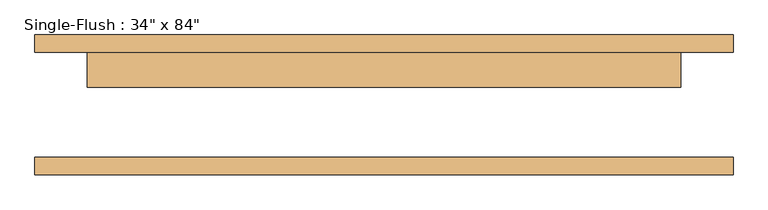
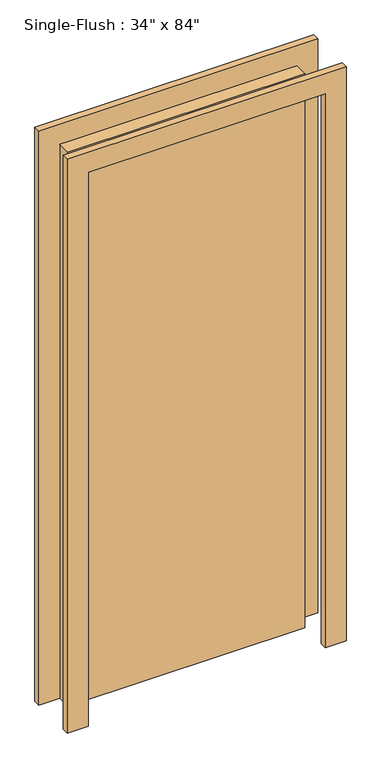
"""IFC4 building model written with IfcOpenShell, lengths in millimetres: door geometry."""

from ifc_helpers import new_model, si_unit, frame, origin, origin_with_axes, place, context, project, spatial, polyline, outline, extrude, source, transform, mapped, element, save


def door_b6e9fca3(model_context):
    return source(origin(), model_context, "Body", "SweptSolid", [
        extrude(outline(polyline([(2209.8, -508.0), (0.0, -508.0), (0.0, -431.8), (2133.6, -431.8), (2133.6, 431.8), (0.0, 431.8), (0.0, 508.0), (2209.8, 508.0), (2209.8, -508.0)])), frame((0.0, 76.2, 0.0), z_axis=(0.0, 1.0, 0.0), x_axis=(0.0, 0.0, 1.0)), (0.0, 0.0, 1.0), 25.4),
        extrude(outline(polyline([(2209.8, 508.0), (2209.8, -508.0), (0.0, -508.0), (0.0, -431.8), (2133.6, -431.8), (2133.6, 431.8), (0.0, 431.8), (0.0, 508.0), (2209.8, 508.0)])), frame((0.0, -101.6, 0.0), z_axis=(0.0, 1.0, 0.0), x_axis=(0.0, 0.0, 1.0)), (0.0, 0.0, 1.0), 25.4),
        extrude(outline(polyline([(431.8, 25.4), (-431.8, 25.4), (-431.8, 76.2), (431.8, 76.2), (431.8, 25.4)])), origin_with_axes(), (0.0, 0.0, 1.0), 2133.6),
    ])


if __name__ == "__main__":
    model = new_model("IFC4")
    model_context = context("Model", 3, world=origin())
    ifc_project = project(units=[si_unit("LENGTHUNIT", "METRE", prefix="MILLI")], contexts=[model_context])
    site = spatial("IfcSite", under=ifc_project)
    building = spatial("IfcBuilding", under=site)
    placement = place(None, origin())
    door_shape = door_b6e9fca3(model_context)
    element("IfcDoor", 1, ObjectType="Single-Flush : 34\" x 84\"", at=placement, inside=building, context=model_context, shape_type="MappedRepresentation", body=[
        mapped(door_shape, transform((0.0, 0.0, 0.0), x_axis=(1.0, 0.0, 0.0), y_axis=(0.0, 1.0, 0.0), z_axis=(0.0, 0.0, 1.0))),
    ])
    save(model, "model.ifc")

# Revit data of these elements
# Type "Single-Flush : 34\" x 84\""
#   Type Mark = "2"
#   Construction Type Id = "MDOOR"
#   Assembly Code = "C1020"
#   Analytic Construction = "Metal"
#   Thickness = 0' - 2"
#   Heat Transfer Coefficient (U) = 0.651978 BTU/(h·ft²·°F)
#   Height = 7' - 0"
#   Trim Projection Ext = 0' - 1"
#   Trim Projection Int = 0' - 1"
#   Trim Width = 0' - 3"
#   Width = 2' - 10"
#   Define Thermal Properties by = 1
#   Door Material = Door - Panel
#   Frame Material = Door - Frame
#   Visual Light Transmittance = 0
#   Solar Heat Gain Coefficient = 0
#   Function = (empty or 0)
#   Wall Closure = (empty or 0)
# Element 1 (IfcDoor, "Single-Flush : 34\" x 84\"")
#   Materials on its faces: "Door - Frame", "Door - Panel"
# Materials
#   "Door - Panel": class "Wood", colour RGB 210 159 95, transparency 0
#   "Door - Frame": colour RGB 118 70 51, transparency 0
